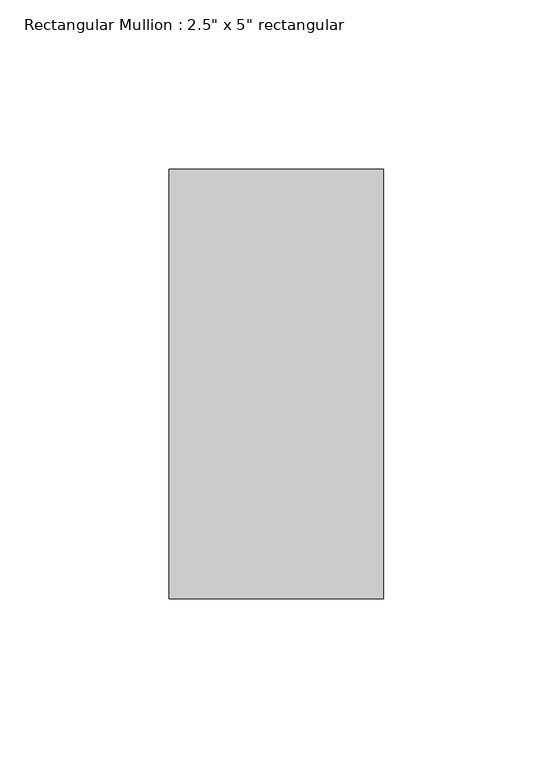
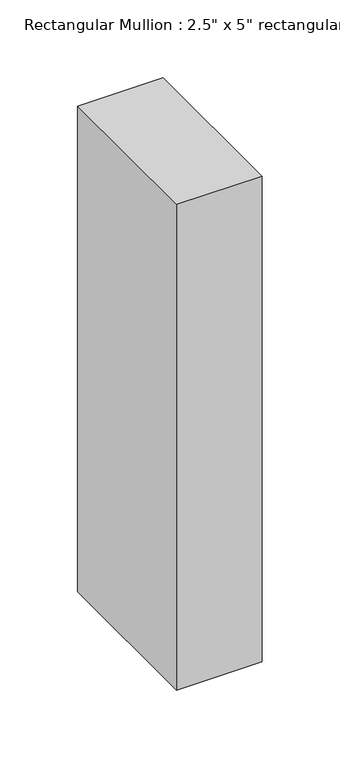
"""IFC4 building model written with IfcOpenShell, lengths in millimetres: member geometry."""

from ifc_helpers import new_model, si_unit, frame, origin, place, context, project, spatial, polyline, outline, extrude, source, transform, mapped, element, save


def member_dfe75557(model_context):
    return source(origin(), model_context, "Body", "SweptSolid", [
        extrude(outline(polyline([(0.0, 63.5), (0.0, -63.5), (-63.5, -63.5), (-63.5, 63.5), (0.0, 63.5)])), frame((0.0, 0.0, -381.0), z_axis=(0.0, 0.0, 1.0), x_axis=(1.0, 0.0, 0.0)), (0.0, 0.0, 1.0), 381.0),
    ])


if __name__ == "__main__":
    model = new_model("IFC4")
    model_context = context("Model", 3, world=origin())
    ifc_project = project(units=[si_unit("LENGTHUNIT", "METRE", prefix="MILLI")], contexts=[model_context])
    site = spatial("IfcSite", under=ifc_project)
    building = spatial("IfcBuilding", under=site)
    placement = place(None, origin())
    member_shape = member_dfe75557(model_context)
    element("IfcMember", 1, ObjectType="Rectangular Mullion : 2.5\" x 5\" rectangular", at=placement, inside=building, context=model_context, shape_type="MappedRepresentation", body=[
        mapped(member_shape, transform((0.0, 0.0, 0.0), x_axis=(1.0, 0.0, 0.0), y_axis=(0.0, 1.0, 0.0), z_axis=(0.0, 0.0, 1.0))),
    ])
    save(model, "model.ifc")

# Revit data of these elements
# Type "Rectangular Mullion : 2.5\" x 5\" rectangular"
#   built-in parameter 1007304 = 0.416667 (stored number, unit not read)
#   built-in parameter 1007301 = 0.104167 (stored number, unit not read)
#   built-in parameter 1007300 = 0.104167 (stored number, unit not read)
# Element 1 (IfcMember, "Rectangular Mullion : 2.5\" x 5\" rectangular")
#   Materials on its faces: "door colour"
# Materials
#   "door colour": class "Generic", colour RGB 120 120 120, transparency 0, Cost = 0
